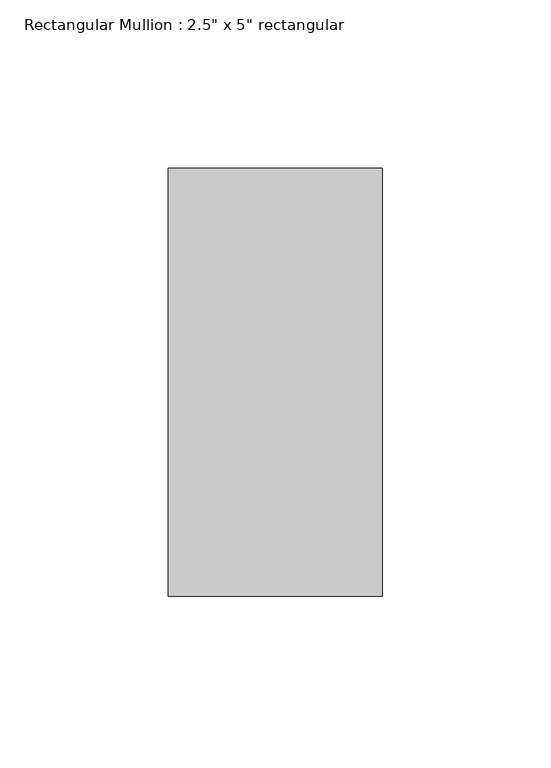
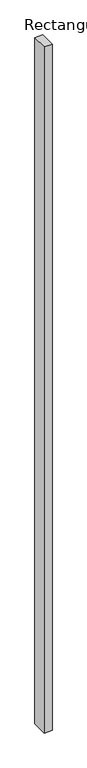
"""IFC4 building model written with IfcOpenShell, lengths in millimetres: member geometry."""

from ifc_helpers import new_model, si_unit, frame, origin, place, context, project, spatial, polyline, outline, extrude, source, transform, mapped, element, save


def member_6fd72b92(model_context):
    return source(origin(), model_context, "Body", "SweptSolid", [
        extrude(outline(polyline([(31.75, 63.5), (31.75, -63.5), (-31.75, -63.5), (-31.75, 63.5), (31.75, 63.5)])), frame((0.0, 0.0, -5793.3288504), z_axis=(0.0, 0.0, 1.0), x_axis=(1.0, 0.0, 0.0)), (0.0, 0.0, 1.0), 5793.3288504),
    ])


if __name__ == "__main__":
    model = new_model("IFC4")
    model_context = context("Model", 3, world=origin())
    ifc_project = project(units=[si_unit("LENGTHUNIT", "METRE", prefix="MILLI")], contexts=[model_context])
    site = spatial("IfcSite", under=ifc_project)
    building = spatial("IfcBuilding", under=site)
    placement = place(None, origin())
    member_shape = member_6fd72b92(model_context)
    element("IfcMember", 1, ObjectType="Rectangular Mullion : 2.5\" x 5\" rectangular", at=placement, inside=building, context=model_context, shape_type="MappedRepresentation", body=[
        mapped(member_shape, transform((0.0, 0.0, 0.0), x_axis=(1.0, 0.0, 0.0), y_axis=(0.0, 1.0, 0.0), z_axis=(0.0, 0.0, 1.0))),
    ])
    save(model, "model.ifc")

# Revit data of these elements
# Type "Rectangular Mullion : 2.5\" x 5\" rectangular"
#   built-in parameter 1007304 = 0.416667 (stored number, unit not read)
#   built-in parameter 1007301 = 0.104167 (stored number, unit not read)
#   built-in parameter 1007300 = 0.104167 (stored number, unit not read)
# Element 1 (IfcMember, "Rectangular Mullion : 2.5\" x 5\" rectangular")
#   Materials on its faces: "Damp-proofing"
# Materials
#   "Damp-proofing": class "Generic", colour RGB 127 127 127, transparency 0, Description = "Damp-proofing", Cost = 0
